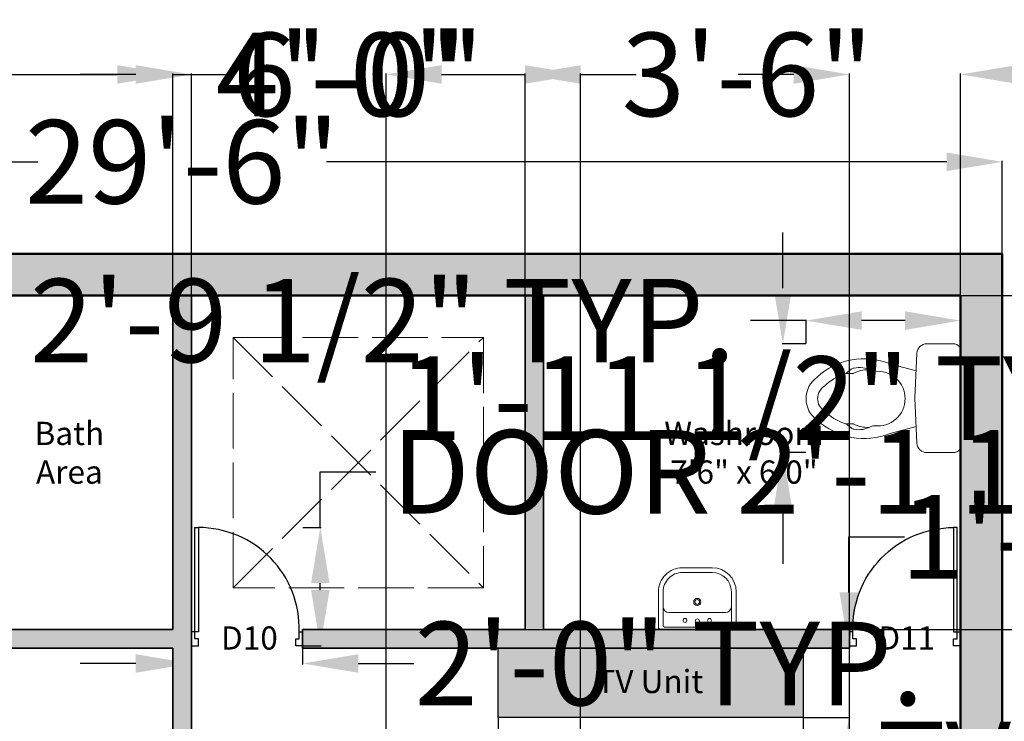
# Model space of a CAD drawing. Units: inches. Extents: x 2796 to 3603, y 978 to 1787.
# Tile 14 of 15: x 3212 to 3425, y 1636 to 1787. Entities that reach past the tile are written whole.
import ezdxf

# ---------------------------------------------------------------- set-up
doc = ezdxf.new("R2010")
doc.units = ezdxf.units.IN
doc.linetypes.add('ACAD_ISO02W100', pattern=[15, 12, -3])
for name, color, linetype, lineweight in [('A-ANNO-DIMS', 7, 'Continuous', 18), ('A-ANNO-TEXT', 7, 'Continuous', 18), ('A-AREA-IDEN', 7, 'Continuous', 18), ('A-DOOR', 6, 'Continuous', 25), ('A-FLOR-CASE', 2, 'Continuous', 25), ('A-FLOR-CASE-PATT', 2, 'Continuous', 13), ('A-FLOR-FIXT', 8, 'Continuous', 18), ('A-FLOR-OVHD', 7, 'ACAD_ISO02W100', 18), ('A-WALL-EXTR-PATT', 1, 'Continuous', 13), ('A-WALL-INTR-PATT', 5, 'Continuous', 13), ('Inner Wall', 5, 'Continuous', 35), ('Outer Wall', 1, 'Continuous', 50)]:
    doc.layers.add(name, color=color, linetype=linetype, lineweight=lineweight)
doc.styles.get("Standard").update_dxf_attribs({"font": 'arial.ttf'})
doc.dimstyles.get("Standard").update_dxf_attribs({"dimtxt": 18, "dimasz": 12, "dimexe": 0.18, "dimexo": 0.0625, "dimgap": 0.09, "dimtad": 0, "dimtih": 1, "dimtoh": 1, "dimdec": 0, "dimzin": 0, "dimdsep": 46, "dimlunit": 3, "dimtxsty": 'Standard', "dimcen": 0.09, "dimadec": 0, "dimazin": 0, "dimtfac": 1, "dimtdec": 0, "dimtofl": 0, "dimtmove": 0, "dimatfit": 3, "dimfxl": 1, "dimtolj": 1, "dimtzin": 0, "dimarcsym": 0})

# ---------------------------------------------------------------- blocks, each defined once
blk = doc.blocks.new('A$C1308471B')
at = {"ltscale": 20}
for p, q in [((0.0354, 0.4793), (0.1495, 0.4793)), ((0, 0.4607), (0, 0.0186)), ((0.2013, 0.2397), (0.1923, 0.4384)), ((0.1957, 0.3639), (0.3109, 0.3953)), ((0.5021, 0.3528), (0.4724, 0.3528)), ((0.4982, 0.3575), (0.4822, 0.3709)), ((0.2013, 0.2397), (0.1923, 0.0409)), ((0.5021, 0.1304), (0.4724, 0.1304)), ((0.1959, 0.1193), (0.3109, 0.0879)), ((0.4982, 0.1257), (0.4822, 0.1123)), ((0.0354, 0), (0.1495, 0))]:
    blk.add_line(p, q, dxfattribs=at)
for centre, radius, start, end in [((0.0354, 0.4328), 0.0465, 90, 136.5269), ((0.1495, 0.4365), 0.0429, 2.5755, 90), ((0.006, 0.4607), 0.006, 136.5269, 180), ((0.4248, 0.1104), 0.3068, 47.4135, 111.7924), ((0.3654, 0.2416), 0.1206, 83.3523, 180), ((0.3823, 0.3868), 0.0255, 263.3523, 298.5742), ((0.4494, 0.2636), 0.1148, 79.3968, 118.5742), ((0.405, 0.2159), 0.153, 63.502, 90.4522), ((0.4658, 0.3513), 0.0255, 50, 79.3968), ((0.5146, 0.377), 0.0255, 230, 251.3881), ((0.5021, 0.3273), 0.0255, 70.3751, 90), ((0.4248, 0.1104), 0.2558, 46.612, 70.3751), ((0.5654, 0.2416), 0.116, 0, 54.7115), ((0.5654, 0.2416), 0.065, 0, 57.2974), ((0.3654, 0.2416), 0.1206, 180, 276.6477), ((0.5654, 0.2416), 0.065, 302.7026, 0), ((0.5654, 0.2416), 0.116, 305.2885, 0), ((0.4248, 0.3728), 0.2558, 289.6249, 313.388), ((0.4248, 0.3728), 0.3068, 248.2076, 312.5865), ((0.405, 0.2673), 0.153, 269.5478, 296.498), ((0.5146, 0.1062), 0.0255, 108.6119, 130), ((0.5021, 0.1559), 0.0255, 270, 289.6249), ((0.3823, 0.0964), 0.0255, 61.4258, 96.6477), ((0.4494, 0.2196), 0.1148, 241.4258, 280.6032), ((0.4658, 0.1319), 0.0255, 280.6032, 310), ((0.006, 0.0186), 0.006, 180, 223.4731), ((0.0354, 0.0465), 0.0465, 223.4731, 270), ((0.1495, 0.0429), 0.0429, 270, 357.4245)]:
    blk.add_arc(centre, radius, start, end, dxfattribs=at)
blk = doc.blocks.new('A$C57EA129C')
for p, q in [((0, 0.4428), (0, 0.1782)), ((0.016, 0.4589), (0.5631, 0.4589)), ((0.0445, 0.441), (0.5346, 0.441)), ((0.5791, 0.4428), (0.5791, 0.1782)), ((0.0356, 0.4321), (0.0356, 0.2896)), ((0.5435, 0.4321), (0.5435, 0.2896)), ((0.0802, 0.3341), (0.499, 0.3341)), ((0.0356, 0.2896), (0.0356, 0.1782)), ((0.5435, 0.2896), (0.5435, 0.1782)), ((0.1782, 0.0356), (0.4009, 0.0356)), ((0.1782, 0), (0.4009, 0))]:
    blk.add_line(p, q)
for centre, radius in [((0.1982, 0.392), 0.0143), ((0.2896, 0.3965), 0.0156), ((0.3809, 0.392), 0.0143), ((0.2896, 0.2545), 0.0267), ((0.2896, 0.2545), 0.0178)]:
    blk.add_circle(centre, radius)
for centre, radius, start, end in [((0.016, 0.4428), 0.016, 90, 180), ((0.0445, 0.4321), 0.00891, 90, 180), ((0.5346, 0.4321), 0.00891, 0, 90), ((0.5631, 0.4428), 0.016, 0, 90), ((0.0802, 0.2896), 0.0445, 90, 180), ((0.499, 0.2896), 0.0445, 0, 90), ((0.1782, 0.1782), 0.1782, 180, 270), ((0.1782, 0.1782), 0.1426, 180, 270), ((0.4009, 0.1782), 0.1782, 270, 0), ((0.4009, 0.1782), 0.1426, 270, 0)]:
    blk.add_arc(centre, radius, start, end)
blk = doc.blocks.new('*D13')
at = {"layer": 'A-ANNO-DIMS', "color": 0, "lineweight": -2, "transparency": 16777216}
for p, q in [((3070.25, 1736.74), (3070.25, 1756.72)), ((3082.25, 1756.54), (3216.09, 1756.54)), ((3412.25, 1756.54), (3278.41, 1756.54)), ((3424.25, 1736.74), (3424.25, 1756.72))]:
    blk.add_line(p, q, dxfattribs=at)
at = {"layer": 'A-ANNO-DIMS', "color": 0, "transparency": 16777216}
for points in [[(3082.25, 1758.54), (3082.25, 1754.54), (3070.25, 1756.54)], [(3412.25, 1758.54), (3412.25, 1754.54), (3424.25, 1756.54)]]:
    blk.add_solid(points, dxfattribs=at)
at = {"layer": 'Defpoints', "color": 0, "transparency": 16777216}
for p in [(3424.25, 1756.54), (3070.25, 1736.68), (3424.25, 1736.68)]:
    blk.add_point(p, dxfattribs=at)
at = {"layer": 'A-ANNO-DIMS', "color": 0, "transparency": 16777216, "insert": (3247.25, 1756.54), "char_height": 18, "attachment_point": 5}
blk.add_mtext('\\A1;29\'-6"', dxfattribs=at)
blk = doc.blocks.new('DOOR-SWING-24IN')
for points in [[(-0.75, -0.7375), (-0.75, 21.7625), (0, 21.7625), (0, -0.7375)], [(-1.5, -3.7375), (0, -3.7375), (0, -2.2375), (-0.75, -2.2375), (-0.75, -0.7375), (-1.5, -0.7375)], [(22.5, -3.7375), (21, -3.7375), (21, -2.2375), (21.75, -2.2375), (21.75, -0.7375), (22.5, -0.7375)]]:
    blk.add_lwpolyline(points, close=True)
blk.add_arc((0, 0), 21.7625, 358.057956, 90)
blk = doc.blocks.new('TV-UNIT-66IN-NOM')
blk.add_lwpolyline([(0, 0), (65.77, 0), (65.77, -15), (0, -15)], close=True)
blk = doc.blocks.new('*D20')
at = {"layer": 'A-ANNO-DIMS', "color": 0, "lineweight": -2, "transparency": 16777216}
for p, q in [((3277.07, 1677.68), (3277.07, 1689.68)), ((3277.07, 1689.68), (3289.07, 1689.68)), ((3273.31, 1677.68), (3277.25, 1677.68)), ((3277.07, 1664.18), (3277.07, 1665.68)), ((3273.31, 1652.18), (3277.25, 1652.18))]:
    blk.add_line(p, q, dxfattribs=at)
at = {"layer": 'A-ANNO-DIMS', "color": 0, "transparency": 16777216}
for points in [[(3275.07, 1665.68), (3279.07, 1665.68), (3277.07, 1677.68)], [(3275.07, 1664.18), (3279.07, 1664.18), (3277.07, 1652.18)]]:
    blk.add_solid(points, dxfattribs=at)
at = {"layer": 'Defpoints', "color": 0, "transparency": 16777216}
for p in [(3273.25, 1677.68), (3277.07, 1677.68), (3273.25, 1652.18)]:
    blk.add_point(p, dxfattribs=at)
at = {"layer": 'A-ANNO-DIMS', "color": 0, "transparency": 16777216, "insert": (3405.76, 1689.68), "char_height": 18, "attachment_point": 5}
blk.add_mtext('\\A1;DOOR 2\'-1 1/2" TYP.', dxfattribs=at)
blk = doc.blocks.new('*D21')
at = {"layer": 'A-ANNO-DIMS', "color": 0, "lineweight": -2, "transparency": 16777216}
for p, q in [((3249.25, 1652.11), (3249.25, 1648.17)), ((3273.25, 1652.11), (3273.25, 1648.17)), ((3237.25, 1648.35), (3225.25, 1648.35)), ((3285.25, 1648.35), (3297.25, 1648.35))]:
    blk.add_line(p, q, dxfattribs=at)
at = {"layer": 'A-ANNO-DIMS', "color": 0, "transparency": 16777216}
for points in [[(3237.25, 1650.35), (3237.25, 1646.35), (3249.25, 1648.35)], [(3285.25, 1650.35), (3285.25, 1646.35), (3273.25, 1648.35)]]:
    blk.add_solid(points, dxfattribs=at)
at = {"layer": 'Defpoints', "color": 0, "transparency": 16777216}
for p in [(3249.25, 1652.18), (3273.25, 1652.18), (3273.25, 1648.35)]:
    blk.add_point(p, dxfattribs=at)
at = {"layer": 'A-ANNO-DIMS', "color": 0, "transparency": 16777216, "insert": (3352.35, 1648.35), "char_height": 18, "attachment_point": 5}
blk.add_mtext('\\A1;2\'-0" TYP.', dxfattribs=at)
blk = doc.blocks.new('*D24')
at = {"layer": 'A-ANNO-DIMS', "color": 0, "lineweight": -2, "transparency": 16777216}
for p, q in [((3381.89, 1722.3), (3369.89, 1722.3)), ((3381.89, 1717.36), (3381.89, 1722.48)), ((3403.25, 1722.3), (3393.89, 1722.3)), ((3415.25, 1717.36), (3415.25, 1722.48))]:
    blk.add_line(p, q, dxfattribs=at)
at = {"layer": 'A-ANNO-DIMS', "color": 0, "transparency": 16777216}
for points in [[(3393.89, 1724.3), (3393.89, 1720.3), (3381.89, 1722.3)], [(3403.25, 1724.3), (3403.25, 1720.3), (3415.25, 1722.3)]]:
    blk.add_solid(points, dxfattribs=at)
at = {"layer": 'Defpoints', "color": 0, "transparency": 16777216}
for p in [(3381.89, 1722.3), (3381.89, 1717.3), (3415.25, 1717.3)]:
    blk.add_point(p, dxfattribs=at)
at = {"layer": 'A-ANNO-DIMS', "color": 0, "transparency": 16777216, "insert": (3269.16, 1722.3), "char_height": 18, "attachment_point": 5}
blk.add_mtext('\\A1;WC 2\'-9 1/2" TYP.', dxfattribs=at)
blk = doc.blocks.new('*D25')
at = {"layer": 'A-ANNO-DIMS', "color": 0, "lineweight": -2, "transparency": 16777216}
for p, q in [((3376.89, 1729.3), (3376.89, 1741.3)), ((3381.83, 1717.3), (3376.71, 1717.3)), ((3381.83, 1693.83), (3376.71, 1693.83)), ((3376.89, 1681.83), (3376.89, 1669.83))]:
    blk.add_line(p, q, dxfattribs=at)
at = {"layer": 'A-ANNO-DIMS', "color": 0, "transparency": 16777216}
for points in [[(3374.89, 1729.3), (3378.89, 1729.3), (3376.89, 1717.3)], [(3374.89, 1681.83), (3378.89, 1681.83), (3376.89, 1693.83)]]:
    blk.add_solid(points, dxfattribs=at)
at = {"layer": 'Defpoints', "color": 0, "transparency": 16777216}
for p in [(3381.89, 1717.3), (3376.89, 1693.83), (3381.89, 1693.83)]:
    blk.add_point(p, dxfattribs=at)
at = {"layer": 'A-ANNO-DIMS', "color": 0, "transparency": 16777216, "insert": (3376.89, 1705.57), "char_height": 18, "attachment_point": 5}
blk.add_mtext('\\A1;1\'-11 1/2" TYP.', dxfattribs=at)
blk = doc.blocks.new('*D28')
at = {"layer": 'A-ANNO-DIMS', "color": 0, "lineweight": -2, "transparency": 16777216}
for p, q in [((3315.48, 1636.61), (3315.48, 1626.63)), ((3381.25, 1636.61), (3381.25, 1626.63)), ((3327.48, 1626.81), (3369.25, 1626.81)), ((3381.25, 1626.81), (3393.25, 1626.81))]:
    blk.add_line(p, q, dxfattribs=at)
at = {"layer": 'A-ANNO-DIMS', "color": 0, "transparency": 16777216}
for points in [[(3327.48, 1628.81), (3327.48, 1624.81), (3315.48, 1626.81)], [(3369.25, 1628.81), (3369.25, 1624.81), (3381.25, 1626.81)]]:
    blk.add_solid(points, dxfattribs=at)
at = {"layer": 'Defpoints', "color": 0, "transparency": 16777216}
for p in [(3315.48, 1636.68), (3381.25, 1636.68), (3381.25, 1626.81)]:
    blk.add_point(p, dxfattribs=at)
at = {"layer": 'A-ANNO-DIMS', "color": 0, "transparency": 16777216, "insert": (3500.81, 1626.81), "char_height": 18, "attachment_point": 5}
blk.add_mtext('\\A1;TV UNIT 5\'-6" TYP.', dxfattribs=at)
blk = doc.blocks.new('*D29')
at = {"layer": 'A-ANNO-DIMS', "color": 0, "lineweight": -2, "transparency": 16777216}
for p, q in [((3391.11, 1663.68), (3391.11, 1675.68)), ((3391.11, 1675.68), (3403.11, 1675.68)), ((3381.31, 1651.68), (3391.29, 1651.68)), ((3381.31, 1636.68), (3391.29, 1636.68)), ((3391.11, 1624.68), (3391.11, 1612.68))]:
    blk.add_line(p, q, dxfattribs=at)
at = {"layer": 'A-ANNO-DIMS', "color": 0, "transparency": 16777216}
for points in [[(3389.11, 1663.68), (3393.11, 1663.68), (3391.11, 1651.68)], [(3389.11, 1624.68), (3393.11, 1624.68), (3391.11, 1636.68)]]:
    blk.add_solid(points, dxfattribs=at)
at = {"layer": 'Defpoints', "color": 0, "transparency": 16777216}
for p in [(3381.25, 1651.68), (3391.11, 1651.68), (3381.25, 1636.68)]:
    blk.add_point(p, dxfattribs=at)
at = {"layer": 'A-ANNO-DIMS', "color": 0, "transparency": 16777216, "insert": (3457.21, 1675.68), "char_height": 18, "attachment_point": 5}
blk.add_mtext('\\A1;1\'-3" TYP.', dxfattribs=at)
blk = doc.blocks.new('*D42')
at = {"layer": 'A-ANNO-DIMS', "color": 0, "lineweight": -2, "transparency": 16777216}
for p, q in [((3291.25, 1311.74), (3291.25, 1775.56)), ((3303.25, 1775.38), (3321.25, 1775.38)), ((3333.25, 1311.74), (3333.25, 1775.56)), ((3333.25, 1775.38), (3345.25, 1775.38))]:
    blk.add_line(p, q, dxfattribs=at)
at = {"layer": 'A-ANNO-DIMS', "color": 0, "transparency": 16777216}
for points in [[(3303.25, 1777.38), (3303.25, 1773.38), (3291.25, 1775.38)], [(3321.25, 1777.38), (3321.25, 1773.38), (3333.25, 1775.38)]]:
    blk.add_solid(points, dxfattribs=at)
at = {"layer": 'Defpoints', "color": 0, "transparency": 16777216}
for p in [(3333.25, 1775.38), (3291.25, 1311.68), (3333.25, 1311.68)]:
    blk.add_point(p, dxfattribs=at)
at = {"layer": 'A-ANNO-DIMS', "color": 0, "transparency": 16777216, "insert": (3369.25, 1775.38), "char_height": 18, "attachment_point": 5}
blk.add_mtext('\\A1;3\'-6"', dxfattribs=at)
blk = doc.blocks.new('*D46')
at = {"layer": 'A-ANNO-DIMS', "color": 0, "lineweight": -2, "transparency": 16777216}
for p, q in [((3197.25, 1727.74), (3197.25, 1775.56)), ((3209.25, 1775.38), (3233.25, 1775.38)), ((3245.25, 1727.74), (3245.25, 1775.56)), ((3245.25, 1775.38), (3257.25, 1775.38))]:
    blk.add_line(p, q, dxfattribs=at)
at = {"layer": 'A-ANNO-DIMS', "color": 0, "transparency": 16777216}
for points in [[(3209.25, 1777.38), (3209.25, 1773.38), (3197.25, 1775.38)], [(3233.25, 1777.38), (3233.25, 1773.38), (3245.25, 1775.38)]]:
    blk.add_solid(points, dxfattribs=at)
at = {"layer": 'Defpoints', "color": 0, "transparency": 16777216}
for p in [(3245.25, 1775.38), (3197.25, 1727.68), (3245.25, 1727.68)]:
    blk.add_point(p, dxfattribs=at)
at = {"layer": 'A-ANNO-DIMS', "color": 0, "transparency": 16777216, "insert": (3281.62, 1775.38), "char_height": 18, "attachment_point": 5}
blk.add_mtext('\\A1;4\'-0"', dxfattribs=at)
blk = doc.blocks.new('*D47')
at = {"layer": 'A-ANNO-DIMS', "color": 0, "lineweight": -2, "transparency": 16777216}
for p, q in [((3237.245499, 1775.37534), (3225.245499, 1775.37534)), ((3249.245499, 1727.73784), (3249.245499, 1775.55534)), ((3321.245499, 1727.73784), (3321.245499, 1775.55534)), ((3333.245499, 1775.37534), (3345.245499, 1775.37534))]:
    blk.add_line(p, q, dxfattribs=at)
at = {"layer": 'A-ANNO-DIMS', "color": 0, "transparency": 16777216}
for points in [[(3237.245499, 1777.37534), (3237.245499, 1773.37534), (3249.245499, 1775.37534)], [(3333.245499, 1777.37534), (3333.245499, 1773.37534), (3321.245499, 1775.37534)]]:
    blk.add_solid(points, dxfattribs=at)
at = {"layer": 'Defpoints', "color": 0, "transparency": 16777216}
for p in [(3321.245499, 1775.37534), (3249.245499, 1727.67534), (3321.245499, 1727.67534)]:
    blk.add_point(p, dxfattribs=at)
at = {"layer": 'A-ANNO-DIMS', "color": 0, "transparency": 16777216, "insert": (3285.245499, 1775.37534), "char_height": 18, "attachment_point": 5}
blk.add_mtext('\\A1;6\'-0"', dxfattribs=at)
blk = doc.blocks.new('*D48')
at = {"layer": 'A-ANNO-DIMS', "color": 0, "lineweight": -2, "transparency": 16777216}
for p, q in [((3321.31, 1727.68), (3463.13, 1727.68)), ((3462.95, 1715.68), (3462.95, 1700.96)), ((3462.95, 1667.68), (3462.95, 1682.4)), ((3321.31, 1655.68), (3463.13, 1655.68))]:
    blk.add_line(p, q, dxfattribs=at)
at = {"layer": 'A-ANNO-DIMS', "color": 0, "transparency": 16777216}
for points in [[(3460.95, 1715.68), (3464.95, 1715.68), (3462.95, 1727.68)], [(3460.95, 1667.68), (3464.95, 1667.68), (3462.95, 1655.68)]]:
    blk.add_solid(points, dxfattribs=at)
at = {"layer": 'Defpoints', "color": 0, "transparency": 16777216}
for p in [(3321.25, 1727.68), (3462.95, 1727.68), (3321.25, 1655.68)]:
    blk.add_point(p, dxfattribs=at)
at = {"layer": 'A-ANNO-DIMS', "color": 0, "transparency": 16777216, "insert": (3462.95, 1691.68), "char_height": 18, "attachment_point": 5}
blk.add_mtext('\\A1;6\'-0"', dxfattribs=at)
blk = doc.blocks.new('*D50')
at = {"layer": 'A-ANNO-DIMS', "color": 0, "lineweight": -2, "transparency": 16777216}
for p, q in [((3379.25, 1775.38), (3367.25, 1775.38)), ((3391.25, 1603.74), (3391.25, 1775.56)), ((3415.25, 1603.74), (3415.25, 1775.56)), ((3427.25, 1775.38), (3439.25, 1775.38))]:
    blk.add_line(p, q, dxfattribs=at)
at = {"layer": 'A-ANNO-DIMS', "color": 0, "transparency": 16777216}
for points in [[(3379.25, 1777.38), (3379.25, 1773.38), (3391.25, 1775.38)], [(3427.25, 1777.38), (3427.25, 1773.38), (3415.25, 1775.38)]]:
    blk.add_solid(points, dxfattribs=at)
at = {"layer": 'Defpoints', "color": 0, "transparency": 16777216}
for p in [(3415.25, 1775.38), (3391.25, 1603.68), (3415.25, 1603.68)]:
    blk.add_point(p, dxfattribs=at)
at = {"layer": 'A-ANNO-DIMS', "color": 0, "transparency": 16777216, "insert": (3463.41, 1775.38), "char_height": 18, "attachment_point": 5}
blk.add_mtext('\\A1;2\'-0"', dxfattribs=at)
blk = doc.blocks.new('*D54')
at = {"layer": 'A-ANNO-DIMS', "color": 0, "lineweight": -2, "transparency": 16777216}
for p, q in [((3379.25, 1775.38), (3367.25, 1775.38)), ((3391.25, 1431.74), (3391.25, 1775.56)), ((3415.25, 1455.74), (3415.25, 1775.56)), ((3427.25, 1775.38), (3439.25, 1775.38))]:
    blk.add_line(p, q, dxfattribs=at)
at = {"layer": 'A-ANNO-DIMS', "color": 0, "transparency": 16777216}
for points in [[(3379.25, 1777.38), (3379.25, 1773.38), (3391.25, 1775.38)], [(3427.25, 1777.38), (3427.25, 1773.38), (3415.25, 1775.38)]]:
    blk.add_solid(points, dxfattribs=at)
at = {"layer": 'Defpoints', "color": 0, "transparency": 16777216}
for p in [(3415.25, 1775.38), (3415.25, 1455.68), (3391.25, 1431.68)]:
    blk.add_point(p, dxfattribs=at)
at = {"layer": 'A-ANNO-DIMS', "color": 0, "transparency": 16777216, "insert": (3463.41, 1775.38), "char_height": 18, "attachment_point": 5}
blk.add_mtext('\\A1;2\'-0"', dxfattribs=at)

msp = doc.modelspace()

# ---------------------------------------------------------------- hatches: boundary and pattern name
at = {"layer": 'A-FLOR-CASE-PATT'}
h = msp.add_hatch(dxfattribs=at)
h.set_pattern_fill('GOST_WOOD', color=256)
h.paths.add_polyline_path([(3127.25, 1727.68), (3079.25, 1727.68), (3079.25, 1703.68), (3127.25, 1703.68)])
h.paths.add_polyline_path([(3245.25, 1629.3), (3230.25, 1629.3), (3230.25, 1563.53), (3245.25, 1563.53)])
h.paths.add_polyline_path([(3381.25, 1651.68), (3315.48, 1651.68), (3315.48, 1636.68), (3381.25, 1636.68)])
h.paths.add_polyline_path([(3415.25, 1603.68), (3391.25, 1603.68), (3391.25, 1507.68), (3415.25, 1507.68)])
h.paths.add_polyline_path([(3199.25, 1407.44), (3184.25, 1407.44), (3184.25, 1353.68), (3199.25, 1353.68)])
h.paths.add_polyline_path([(3199.25, 1455.68), (3127.25, 1455.68), (3127.25, 1431.68), (3199.25, 1431.68)])
h.paths.add_polyline_path([(3223.25, 1244.56), (3208.25, 1244.56), (3208.25, 1178.79), (3223.25, 1178.79)])
h.paths.add_polyline_path([(3093.36, 1710.13), (3112.68, 1710.13), (3112.68, 1720.81), (3093.36, 1720.81)], flags=24)
h.paths.add_polyline_path([(3232.57, 1610.37), (3232.57, 1583.04), (3243.25, 1583.04), (3243.25, 1610.37)], flags=24)
h.paths.add_polyline_path([(3334.41, 1639), (3361.73, 1639), (3361.73, 1649.68), (3334.41, 1649.68)], flags=24)
h.paths.add_polyline_path([(3398.2, 1565.36), (3398.2, 1546.04), (3408.87, 1546.04), (3408.87, 1565.36)], flags=24)
h.paths.add_polyline_path([(3186.57, 1394.51), (3186.57, 1367.19), (3197.25, 1367.19), (3197.25, 1394.51)], flags=24)
h.paths.add_polyline_path([(3153.56, 1438.63), (3172.88, 1438.63), (3172.88, 1449.3), (3153.56, 1449.3)], flags=24)
h.paths.add_polyline_path([(3210.57, 1225.63), (3210.57, 1198.3), (3221.25, 1198.3), (3221.25, 1225.63)], flags=24)
at = {"layer": 'A-WALL-EXTR-PATT'}
h = msp.add_hatch(color=256, dxfattribs=at)
h.dxf.hatch_style = 1
h.paths.add_polyline_path([(3424.25, 1736.68), (3070.25, 1736.68), (3070.25, 1106.68), (3227.25, 1106.68), (3227.25, 1115.68), (3226.75, 1115.68), (3223.75, 1115.68), (3079.25, 1115.68), (3079.25, 1727.68), (3127.25, 1727.68), (3415.25, 1727.68), (3415.25, 1188.68), (3424.25, 1188.68)])
h.paths.add_polyline_path([(3291.25, 1032.68), (3074.25, 1032.68), (3074.25, 1106.68), (3070.25, 1106.68), (3070.25, 1028.68), (3291.25, 1028.68)])
h.paths.add_polyline_path([(3291.25, 1115.68), (3281.25, 1115.68), (3281.25, 1106.68), (3291.25, 1106.68)], flags=17)
h.paths.add_polyline_path([(3301.25, 1037.68), (3291.25, 1037.68), (3291.25, 1028.68), (3301.25, 1028.68)])
h.paths.add_polyline_path([(3424.25, 1037.68), (3414.25, 1037.68), (3414.25, 1028.68), (3424.25, 1028.68)])
h.paths.add_polyline_path([(3424.25, 1188.68), (3420.25, 1188.68), (3420.25, 1037.68), (3424.25, 1037.68)])
at = {"layer": 'A-WALL-INTR-PATT'}
h = msp.add_hatch(color=256, dxfattribs=at)
h.dxf.hatch_style = 1
h.paths.add_polyline_path([(3249.25, 1727.68), (3245.25, 1727.68), (3245.25, 1655.68), (3103.25, 1655.68), (3103.25, 1651.68), (3245.25, 1651.68), (3245.25, 1503.68), (3249.25, 1503.68)])
h.paths.add_polyline_path([(3131.25, 1727.68), (3127.25, 1727.68), (3127.25, 1703.68), (3127.25, 1679.68), (3131.25, 1679.68)], flags=17)
h.paths.add_polyline_path([(3391.25, 1655.68), (3325.25, 1655.68), (3325.25, 1727.68), (3321.25, 1727.68), (3321.25, 1655.68), (3273.25, 1655.68), (3273.25, 1651.68), (3391.25, 1651.68)])
h.paths.add_polyline_path([(3203.25, 1459.68), (3079.25, 1459.68), (3079.25, 1455.68), (3199.25, 1455.68), (3199.25, 1431.68), (3199.25, 1347.68), (3203.25, 1347.68)])
h.paths.add_polyline_path([(3209.25, 1507.68), (3079.25, 1507.68), (3079.25, 1503.68), (3209.25, 1503.68)])
h.paths.add_polyline_path([(3415.25, 1507.68), (3285.25, 1507.68), (3285.25, 1503.68), (3415.25, 1503.68)])
h.paths.add_polyline_path([(3415.25, 1459.68), (3333.25, 1459.68), (3333.25, 1455.68), (3415.25, 1455.68)])
h.paths.add_polyline_path([(3291.25, 1311.68), (3287.25, 1311.68), (3287.25, 1192.68), (3227.25, 1192.68), (3227.25, 1267.68), (3263.25, 1267.68), (3263.25, 1271.68), (3223.25, 1271.68), (3223.25, 1151.68), (3227.25, 1151.68), (3227.25, 1188.68), (3291.25, 1188.68)])
h.paths.add_polyline_path([(3227.25, 1311.68), (3079.25, 1311.68), (3079.25, 1307.68), (3227.25, 1307.68)])

# ---------------------------------------------------------------- linework, layer by layer
at = {"layer": 'A-FLOR-OVHD'}
for p, q in [((3258.25, 1718.68), (3312.25, 1664.68)), ((3258.25, 1664.68), (3312.25, 1718.68))]:
    msp.add_line(p, q, dxfattribs=at)
msp.add_lwpolyline([(3258.25, 1718.68), (3312.25, 1718.68), (3312.25, 1664.68), (3258.25, 1664.68)], close=True, dxfattribs=at)
at = {"layer": 'Inner Wall'}
for p, q in [((3245.25, 1655.68), (3245.25, 1727.68)), ((3249.25, 1503.68), (3249.25, 1727.68)), ((3321.25, 1727.68), (3321.25, 1655.68)), ((3325.25, 1727.68), (3325.25, 1655.68)), ((3103.25, 1655.68), (3245.25, 1655.68)), ((3273.25, 1655.68), (3321.25, 1655.68)), ((3273.25, 1651.68), (3273.25, 1655.68)), ((3325.25, 1655.68), (3391.25, 1655.68)), ((3391.25, 1655.68), (3391.25, 1651.68)), ((3103.25, 1651.68), (3245.25, 1651.68)), ((3245.25, 1503.68), (3245.25, 1651.68)), ((3273.25, 1651.68), (3391.25, 1651.68))]:
    msp.add_line(p, q, dxfattribs=at)
at = {"layer": 'Outer Wall'}
for p, q in [((3070.25, 1736.68), (3424.25, 1736.68)), ((3424.25, 1736.68), (3424.25, 1028.68)), ((3079.25, 1727.68), (3415.25, 1727.68)), ((3415.25, 1727.68), (3415.25, 1188.68))]:
    msp.add_line(p, q, dxfattribs=at)

# ---------------------------------------------------------------- block references
at = {"layer": 'A-DOOR'}
msp.add_blockref('DOOR-SWING-24IN', (3250.75, 1655.91), dxfattribs=at)
at = {"layer": 'A-DOOR', "extrusion": (0, 0, -1), "zscale": -1}
msp.add_blockref('DOOR-SWING-24IN', (-3413.75, 1655.91), dxfattribs=at)
at = {"layer": 'A-FLOR-CASE'}
msp.add_blockref('TV-UNIT-66IN-NOM', (3315.48, 1651.68), dxfattribs=at)
at = {"layer": 'A-FLOR-FIXT', "rotation": 180}
for name, p, xscale, yscale, zscale in [('A$C1308471B', (3415.25, 1717.3), 48.95497407897215, 48.95497407897215, 48.95497407897215), ('A$C57EA129C', (3366.81, 1669), 28.98333223671166, 28.98333223671166, 28.98333223671166)]:
    msp.add_blockref(name, p, dxfattribs=dict(at, xscale=xscale, yscale=yscale, zscale=zscale))

# ---------------------------------------------------------------- texts
at = {"layer": 'A-ANNO-TEXT', "char_height": 5, "attachment_point": 3}
for s, width, insert in [('\\pxqc;{\\fTimes New Roman|b0|i0|c0|p18;D10}', 15.6741, (3269.6, 1656.35)), ('\\pxqc;{\\fTimes New Roman|b0|i0|c0|p18;D11}', 15.6741, (3411.47, 1656.35)), ('\\pxqc;{\\fTimes New Roman|b0|i0|c0|p18;TV Unit}', 35.2337, (3365.8, 1646.97))]:
    msp.add_mtext_dynamic_manual_height_columns(s, width=width, gutter_width=12.5, heights=[0], dxfattribs=dict(at, insert=insert))
at = {"layer": 'A-AREA-IDEN', "char_height": 5, "attachment_point": 3}
for s, insert in [('\\pxqc;{\\fTimes New Roman|b0|i0|c0|p18;Bath\\PArea}', (3240.53, 1700.47)), ('\\pxqc;{\\fTimes New Roman|b0|i0|c0|p18;Washroom\\P7\'6" x 6\'0"}', (3386.11, 1700.47))]:
    msp.add_mtext_dynamic_manual_height_columns(s, width=35.2337, gutter_width=12.5, heights=[0], dxfattribs=dict(at, insert=insert))

# ---------------------------------------------------------------- dimensions: what is measured, and where the dimension line sits
at = {"layer": 'A-ANNO-DIMS'}
for base, p1, p2, override, picture, middle in [((3245.25, 1775.38), (3197.25, 1727.68), (3245.25, 1727.68), {"dimdec": 1, "dimlfac": 1, "dimrnd": 0, "dimzin": 1, "dimdsep": 46, "dimlunit": 4, "dimfrac": 2}, '*D46', (3281.62, 1775.38)), ((3321.25, 1775.38), (3249.25, 1727.68), (3321.25, 1727.68), {"dimdec": 1, "dimlfac": 1, "dimrnd": 0, "dimzin": 1, "dimdsep": 46, "dimlunit": 4, "dimfrac": 2}, '*D47', (3285.25, 1775.38)), ((3333.25, 1775.38), (3291.25, 1311.68), (3333.25, 1311.68), {"dimdec": 1, "dimlfac": 1, "dimrnd": 0, "dimzin": 1, "dimdsep": 46, "dimlunit": 4, "dimfrac": 2}, '*D42', (3369.25, 1775.38)), ((3415.25, 1775.38), (3391.25, 1603.68), (3415.25, 1603.68), {"dimdec": 1, "dimlfac": 1, "dimrnd": 0, "dimzin": 1, "dimdsep": 46, "dimlunit": 4, "dimfrac": 2}, '*D50', (3463.41, 1775.38)), ((3415.25, 1775.38), (3391.25, 1431.68), (3415.25, 1455.68), {"dimdec": 1, "dimlfac": 1, "dimrnd": 0, "dimzin": 1, "dimdsep": 46, "dimlunit": 4, "dimfrac": 2}, '*D54', (3463.41, 1775.38)), ((3424.25, 1756.54), (3070.25, 1736.68), (3424.25, 1736.68), {"dimclrd": 0, "dimclre": 0, "dimclrt": 0}, '*D13', (3247.25, 1756.54))]:
    dim = msp.add_linear_dim(base=base, p1=p1, p2=p2, dimstyle='Standard', override=override, dxfattribs=at)
    dim.commit()
    dim.dimension.update_dxf_attribs({"geometry": picture, "text_midpoint": middle})
for base, p1, p2, angle, text, picture, middle in [((3381.89, 1722.3), (3415.25, 1717.3), (3381.89, 1717.3), 180, 'WC <> TYP.', '*D24', (3269.16, 1722.3)), ((3376.89, 1693.83), (3381.89, 1717.3), (3381.89, 1693.83), 270, '<> TYP.', '*D25', (3376.89, 1705.57)), ((3277.07, 1677.68), (3273.25, 1652.18), (3273.25, 1677.68), 90, 'DOOR <> TYP.', '*D20', (3405.76, 1689.68)), ((3391.11, 1651.68), (3381.25, 1636.68), (3381.25, 1651.68), 90, '<> TYP.', '*D29', (3457.21, 1675.68))]:
    dim = msp.add_linear_dim(base=base, p1=p1, p2=p2, angle=angle, text=text, dimstyle='Standard', override={"dimdec": 1, "dimlfac": 1, "dimrnd": 0, "dimzin": 1, "dimdsep": 46, "dimlunit": 4, "dimfrac": 2}, dxfattribs=at)
    dim.commit()
    dim.dimension.update_dxf_attribs({"geometry": picture, "text_midpoint": middle})
dim = msp.add_linear_dim(base=(3462.95, 1727.68), p1=(3321.25, 1655.68), p2=(3321.25, 1727.68), angle=90, dimstyle='Standard', override={"dimdec": 1, "dimlfac": 1, "dimrnd": 0, "dimzin": 1, "dimdsep": 46, "dimlunit": 4, "dimfrac": 2}, dxfattribs=at)
dim.commit()
dim.dimension.update_dxf_attribs({"geometry": '*D48', "text_midpoint": (3462.95, 1691.68)})
for base, p1, p2, text, picture, middle in [((3381.25, 1626.81), (3315.48, 1636.68), (3381.25, 1636.68), 'TV UNIT <> TYP.', '*D28', (3500.81, 1626.81)), ((3273.25, 1648.35), (3249.25, 1652.18), (3273.25, 1652.18), '<> TYP.', '*D21', (3352.35, 1648.35))]:
    dim = msp.add_linear_dim(base=base, p1=p1, p2=p2, text=text, dimstyle='Standard', override={"dimdec": 1, "dimlfac": 1, "dimrnd": 0, "dimzin": 1, "dimdsep": 46, "dimlunit": 4, "dimfrac": 2}, dxfattribs=at)
    dim.commit()
    dim.dimension.update_dxf_attribs({"geometry": picture, "text_midpoint": middle})

doc.saveas('drawing.dxf')
